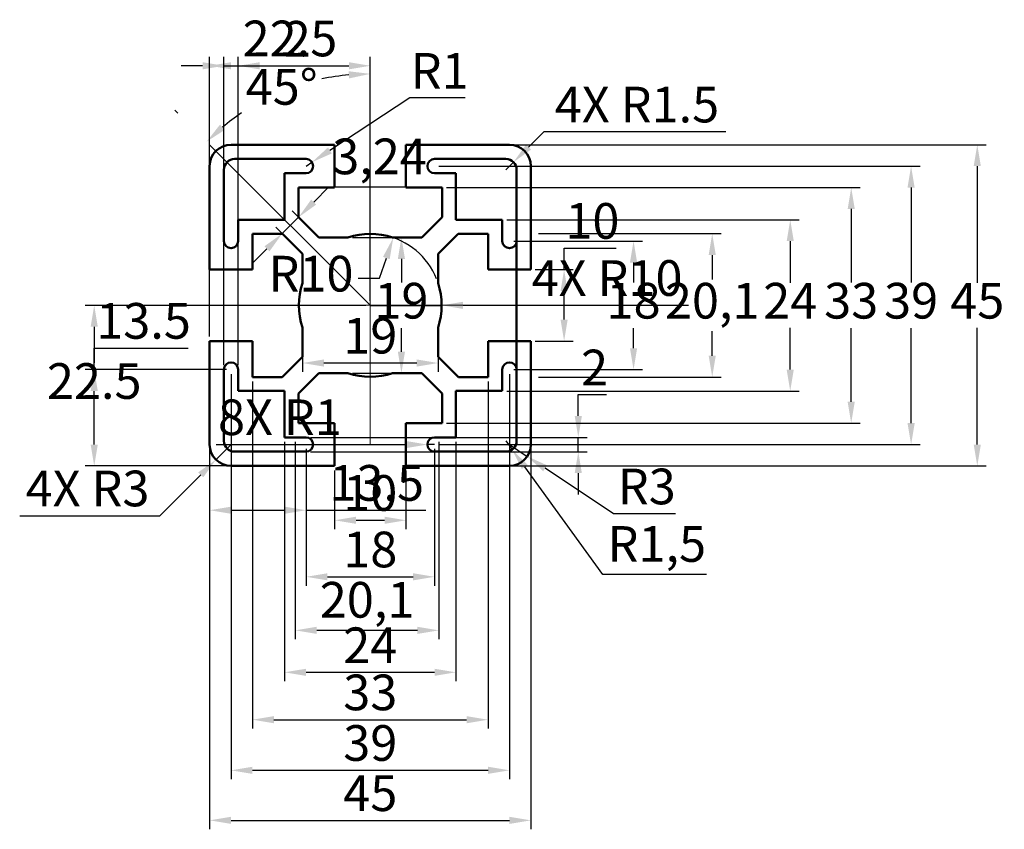
# Model space of a CAD drawing. Units: millimetres. Extents: x 19 to 157, y -26 to 87.
import ezdxf

# ---------------------------------------------------------------- set-up
doc = ezdxf.new("R2010")
doc.units = ezdxf.units.MM
doc.linetypes.add('CENTER', pattern=[50.8, 31.75, -6.35, 6.35, -6.35])
for name, color, linetype, lineweight in [('M-CNTR', 1, 'CENTER', 18), ('M-DIMS', 2, 'Continuous', 25), ('M-OUTL', 7, 'Continuous', 50)]:
    doc.layers.add(name, color=color, linetype=linetype, lineweight=lineweight)
doc.styles.get("Standard").update_dxf_attribs({"font": 'arial.ttf'})
doc.dimstyles.new('ISO-25', dxfattribs={"dimtxt": 5, "dimasz": 3, "dimexe": 1.25, "dimexo": 0.625, "dimtad": 1, "dimtih": 1, "dimtoh": 1, "dimtxsty": 'Standard', "dimcen": 2.5, "dimadec": 0, "dimazin": 0, "dimtfac": 1, "dimtmove": 0, "dimatfit": 3, "dimfxl": 1, "dimarcsym": 0})

# ---------------------------------------------------------------- blocks, each defined once
blk = doc.blocks.new('*D1')
at = {"layer": 'Defpoints', "color": 0, "transparency": 16777216}
for p in [(63.57, 24.73), (73.57, 24.73), (73.57, 17.12)]:
    blk.add_point(p, dxfattribs=at)
at = {"layer": 'M-DIMS', "color": 0, "lineweight": -2, "transparency": 16777216}
for p, q in [((63.57, 24.11), (63.57, 15.87)), ((73.57, 24.11), (73.57, 15.87)), ((66.57, 17.12), (70.57, 17.12))]:
    blk.add_line(p, q, dxfattribs=at)
at = {"layer": 'M-DIMS', "color": 0, "transparency": 16777216}
for points in [[(66.57, 17.62), (66.57, 16.62), (63.57, 17.12)], [(70.57, 17.62), (70.57, 16.62), (73.57, 17.12)]]:
    blk.add_solid(points, dxfattribs=at)
at = {"layer": 'M-DIMS', "color": 0, "transparency": 16777216, "insert": (68.57, 20.3), "char_height": 5, "attachment_point": 5}
blk.add_mtext('10', dxfattribs=at)
blk = doc.blocks.new('*D2')
at = {"layer": 'Defpoints', "color": 0, "transparency": 16777216}
for p in [(59.57, 27.73), (77.57, 27.73), (77.57, 9.2)]:
    blk.add_point(p, dxfattribs=at)
at = {"layer": 'M-DIMS', "color": 0, "lineweight": -2, "transparency": 16777216}
for p, q in [((59.57, 27.11), (59.57, 7.95)), ((77.57, 27.11), (77.57, 7.95)), ((62.57, 9.2), (74.57, 9.2))]:
    blk.add_line(p, q, dxfattribs=at)
at = {"layer": 'M-DIMS', "color": 0, "transparency": 16777216}
for points in [[(62.57, 9.7), (62.57, 8.7), (59.57, 9.2)], [(74.57, 9.7), (74.57, 8.7), (77.57, 9.2)]]:
    blk.add_solid(points, dxfattribs=at)
at = {"layer": 'M-DIMS', "color": 0, "transparency": 16777216, "insert": (68.57, 12.38), "char_height": 5, "attachment_point": 5}
blk.add_mtext('18', dxfattribs=at)
blk = doc.blocks.new('*D3')
at = {"layer": 'Defpoints', "color": 0, "transparency": 16777216}
for p in [(56.57, 28.73), (80.57, 28.73), (80.57, -4.18)]:
    blk.add_point(p, dxfattribs=at)
at = {"layer": 'M-DIMS', "color": 0, "lineweight": -2, "transparency": 16777216}
for p, q in [((56.57, 28.11), (56.57, -5.43)), ((80.57, 28.11), (80.57, -5.43)), ((59.57, -4.18), (77.57, -4.18))]:
    blk.add_line(p, q, dxfattribs=at)
at = {"layer": 'M-DIMS', "color": 0, "transparency": 16777216}
for points in [[(59.57, -3.68), (59.57, -4.68), (56.57, -4.18)], [(77.57, -3.68), (77.57, -4.68), (80.57, -4.18)]]:
    blk.add_solid(points, dxfattribs=at)
at = {"layer": 'M-DIMS', "color": 0, "transparency": 16777216, "insert": (68.57, -1.04), "char_height": 5, "attachment_point": 5}
blk.add_mtext('24', dxfattribs=at)
blk = doc.blocks.new('*D4')
at = {"layer": 'Defpoints', "color": 0, "transparency": 16777216}
for p in [(58.07, 28.73), (78.17, 28.73), (58.07, 1.7)]:
    blk.add_point(p, dxfattribs=at)
at = {"layer": 'M-DIMS', "color": 0, "lineweight": -2, "transparency": 16777216}
for p, q in [((58.07, 28.11), (58.07, 0.45)), ((78.17, 28.11), (78.17, 0.45)), ((75.17, 1.7), (61.07, 1.7))]:
    blk.add_line(p, q, dxfattribs=at)
at = {"layer": 'M-DIMS', "color": 0, "transparency": 16777216}
for points in [[(61.07, 2.2), (61.07, 1.2), (58.07, 1.7)], [(75.17, 2.2), (75.17, 1.2), (78.17, 1.7)]]:
    blk.add_solid(points, dxfattribs=at)
at = {"layer": 'M-DIMS', "color": 0, "transparency": 16777216, "insert": (68.12, 5.33), "char_height": 5, "attachment_point": 5}
blk.add_mtext('20,1', dxfattribs=at)
blk = doc.blocks.new('*D5')
at = {"layer": 'Defpoints', "color": 0, "transparency": 16777216}
for p in [(52.07, 37.18), (85.07, 37.18), (85.07, -10.82)]:
    blk.add_point(p, dxfattribs=at)
at = {"layer": 'M-DIMS', "color": 0, "lineweight": -2, "transparency": 16777216}
for p, q in [((52.07, 36.56), (52.07, -12.07)), ((85.07, 36.56), (85.07, -12.07)), ((55.07, -10.82), (82.07, -10.82))]:
    blk.add_line(p, q, dxfattribs=at)
at = {"layer": 'M-DIMS', "color": 0, "transparency": 16777216}
for points in [[(55.07, -10.32), (55.07, -11.32), (52.07, -10.82)], [(82.07, -10.32), (82.07, -11.32), (85.07, -10.82)]]:
    blk.add_solid(points, dxfattribs=at)
at = {"layer": 'M-DIMS', "color": 0, "transparency": 16777216, "insert": (68.57, -7.64), "char_height": 5, "attachment_point": 5}
blk.add_mtext('33', dxfattribs=at)
blk = doc.blocks.new('*D6')
at = {"layer": 'Defpoints', "color": 0, "transparency": 16777216}
for p in [(49.07, 38.23), (88.07, 38.23), (88.07, -17.91)]:
    blk.add_point(p, dxfattribs=at)
at = {"layer": 'M-DIMS', "color": 0, "lineweight": -2, "transparency": 16777216}
for p, q in [((49.07, 37.61), (49.07, -19.16)), ((88.07, 37.61), (88.07, -19.16)), ((52.07, -17.91), (85.07, -17.91))]:
    blk.add_line(p, q, dxfattribs=at)
at = {"layer": 'M-DIMS', "color": 0, "transparency": 16777216}
for points in [[(52.07, -17.41), (52.07, -18.41), (49.07, -17.91)], [(85.07, -17.41), (85.07, -18.41), (88.07, -17.91)]]:
    blk.add_solid(points, dxfattribs=at)
at = {"layer": 'M-DIMS', "color": 0, "transparency": 16777216, "insert": (68.57, -14.73), "char_height": 5, "attachment_point": 5}
blk.add_mtext('39', dxfattribs=at)
blk = doc.blocks.new('*D7')
at = {"layer": 'Defpoints', "color": 0, "transparency": 16777216}
for p in [(46.07, 27.73), (91.07, 27.73), (91.07, -24.92)]:
    blk.add_point(p, dxfattribs=at)
at = {"layer": 'M-DIMS', "color": 0, "lineweight": -2, "transparency": 16777216}
for p, q in [((46.07, 27.11), (46.07, -26.17)), ((91.07, 27.11), (91.07, -26.17)), ((49.07, -24.92), (88.07, -24.92))]:
    blk.add_line(p, q, dxfattribs=at)
at = {"layer": 'M-DIMS', "color": 0, "transparency": 16777216}
for points in [[(49.07, -24.42), (49.07, -25.42), (46.07, -24.92)], [(88.07, -24.42), (88.07, -25.42), (91.07, -24.92)]]:
    blk.add_solid(points, dxfattribs=at)
at = {"layer": 'M-DIMS', "color": 0, "transparency": 16777216, "insert": (68.57, -21.76), "char_height": 5, "attachment_point": 5}
blk.add_mtext('45', dxfattribs=at)
blk = doc.blocks.new('*D8')
at = {"layer": 'Defpoints', "color": 0, "transparency": 16777216}
for p in [(91.07, 52.23), (95.72, 52.23), (91.07, 42.23)]:
    blk.add_point(p, dxfattribs=at)
at = {"layer": 'M-DIMS', "color": 0, "lineweight": -2, "transparency": 16777216}
for p, q in [((95.72, 52.23), (95.72, 55.23)), ((95.72, 55.23), (103.02, 55.23)), ((91.69, 52.23), (96.97, 52.23)), ((95.72, 45.23), (95.72, 49.23)), ((91.69, 42.23), (96.97, 42.23))]:
    blk.add_line(p, q, dxfattribs=at)
at = {"layer": 'M-DIMS', "color": 0, "transparency": 16777216}
for points in [[(95.22, 49.23), (96.22, 49.23), (95.72, 52.23)], [(95.22, 45.23), (96.22, 45.23), (95.72, 42.23)]]:
    blk.add_solid(points, dxfattribs=at)
at = {"layer": 'M-DIMS', "color": 0, "transparency": 16777216, "insert": (99.68, 58.41), "char_height": 5, "attachment_point": 5}
blk.add_mtext('10', dxfattribs=at)
blk = doc.blocks.new('*D9')
at = {"layer": 'Defpoints', "color": 0, "transparency": 16777216}
for p in [(88.07, 56.23), (105.45, 56.23), (88.07, 38.23)]:
    blk.add_point(p, dxfattribs=at)
at = {"layer": 'M-DIMS', "color": 0, "lineweight": -2, "transparency": 16777216}
for p, q in [((88.69, 56.23), (106.7, 56.23)), ((105.45, 53.23), (105.45, 50.41)), ((105.45, 41.23), (105.45, 44.05)), ((88.69, 38.23), (106.7, 38.23))]:
    blk.add_line(p, q, dxfattribs=at)
at = {"layer": 'M-DIMS', "color": 0, "transparency": 16777216}
for points in [[(104.95, 53.23), (105.95, 53.23), (105.45, 56.23)], [(104.95, 41.23), (105.95, 41.23), (105.45, 38.23)]]:
    blk.add_solid(points, dxfattribs=at)
at = {"layer": 'M-DIMS', "color": 0, "transparency": 16777216, "insert": (105.45, 47.23), "char_height": 5, "attachment_point": 5}
blk.add_mtext('18', dxfattribs=at)
blk = doc.blocks.new('*D10')
at = {"layer": 'Defpoints', "color": 0, "transparency": 16777216}
for p in [(91.51, 57.28), (116.47, 57.28), (91.51, 37.18)]:
    blk.add_point(p, dxfattribs=at)
at = {"layer": 'M-DIMS', "color": 0, "lineweight": -2, "transparency": 16777216}
for p, q in [((92.14, 57.28), (117.72, 57.28)), ((116.47, 54.28), (116.47, 50.86)), ((116.47, 40.18), (116.47, 43.6)), ((92.14, 37.18), (117.72, 37.18))]:
    blk.add_line(p, q, dxfattribs=at)
at = {"layer": 'M-DIMS', "color": 0, "transparency": 16777216}
for points in [[(115.97, 54.28), (116.97, 54.28), (116.47, 57.28)], [(115.97, 40.18), (116.97, 40.18), (116.47, 37.18)]]:
    blk.add_solid(points, dxfattribs=at)
at = {"layer": 'M-DIMS', "color": 0, "transparency": 16777216, "insert": (116.47, 47.23), "char_height": 5, "attachment_point": 5}
blk.add_mtext('20,1', dxfattribs=at)
blk = doc.blocks.new('*D11')
at = {"layer": 'Defpoints', "color": 0, "transparency": 16777216}
for p in [(87.07, 59.23), (127.4, 59.23), (87.07, 35.23)]:
    blk.add_point(p, dxfattribs=at)
at = {"layer": 'M-DIMS', "color": 0, "lineweight": -2, "transparency": 16777216}
for p, q in [((87.69, 59.23), (128.65, 59.23)), ((127.4, 56.23), (127.4, 50.37)), ((127.4, 38.23), (127.4, 44.1)), ((87.69, 35.23), (128.65, 35.23))]:
    blk.add_line(p, q, dxfattribs=at)
at = {"layer": 'M-DIMS', "color": 0, "transparency": 16777216}
for points in [[(126.9, 56.23), (127.9, 56.23), (127.4, 59.23)], [(126.9, 38.23), (127.9, 38.23), (127.4, 35.23)]]:
    blk.add_solid(points, dxfattribs=at)
at = {"layer": 'M-DIMS', "color": 0, "transparency": 16777216, "insert": (127.4, 47.23), "char_height": 5, "attachment_point": 5}
blk.add_mtext('24', dxfattribs=at)
blk = doc.blocks.new('*D12')
at = {"layer": 'Defpoints', "color": 0, "transparency": 16777216}
for p in [(78.62, 63.73), (135.94, 63.73), (78.62, 30.73)]:
    blk.add_point(p, dxfattribs=at)
at = {"layer": 'M-DIMS', "color": 0, "lineweight": -2, "transparency": 16777216}
for p, q in [((79.24, 63.73), (137.19, 63.73)), ((135.94, 60.73), (135.94, 50.41)), ((135.94, 33.73), (135.94, 44.05)), ((79.24, 30.73), (137.19, 30.73))]:
    blk.add_line(p, q, dxfattribs=at)
at = {"layer": 'M-DIMS', "color": 0, "transparency": 16777216}
for points in [[(135.44, 60.73), (136.44, 60.73), (135.94, 63.73)], [(135.44, 33.73), (136.44, 33.73), (135.94, 30.73)]]:
    blk.add_solid(points, dxfattribs=at)
at = {"layer": 'M-DIMS', "color": 0, "transparency": 16777216, "insert": (135.94, 47.23), "char_height": 5, "attachment_point": 5}
blk.add_mtext('33', dxfattribs=at)
blk = doc.blocks.new('*D13')
at = {"layer": 'Defpoints', "color": 0, "transparency": 16777216}
for p in [(77.57, 66.73), (77.57, 27.73), (144.33, 27.73)]:
    blk.add_point(p, dxfattribs=at)
at = {"layer": 'M-DIMS', "color": 0, "lineweight": -2, "transparency": 16777216}
for p, q in [((78.19, 66.73), (145.58, 66.73)), ((144.33, 63.73), (144.33, 50.41)), ((144.33, 30.73), (144.33, 44.05)), ((78.19, 27.73), (145.58, 27.73))]:
    blk.add_line(p, q, dxfattribs=at)
at = {"layer": 'M-DIMS', "color": 0, "transparency": 16777216}
for points in [[(143.83, 63.73), (144.83, 63.73), (144.33, 66.73)], [(143.83, 30.73), (144.83, 30.73), (144.33, 27.73)]]:
    blk.add_solid(points, dxfattribs=at)
at = {"layer": 'M-DIMS', "color": 0, "transparency": 16777216, "insert": (144.33, 47.23), "char_height": 5, "attachment_point": 5}
blk.add_mtext('39', dxfattribs=at)
blk = doc.blocks.new('*D14')
at = {"layer": 'Defpoints', "color": 0, "transparency": 16777216}
for p in [(88.07, 69.73), (88.07, 24.73), (153.6, 24.73)]:
    blk.add_point(p, dxfattribs=at)
at = {"layer": 'M-DIMS', "color": 0, "lineweight": -2, "transparency": 16777216}
for p, q in [((88.69, 69.73), (154.85, 69.73)), ((153.6, 66.73), (153.6, 50.4)), ((153.6, 27.73), (153.6, 44.06)), ((88.69, 24.73), (154.85, 24.73))]:
    blk.add_line(p, q, dxfattribs=at)
at = {"layer": 'M-DIMS', "color": 0, "transparency": 16777216}
for points in [[(153.1, 66.73), (154.1, 66.73), (153.6, 69.73)], [(153.1, 27.73), (154.1, 27.73), (153.6, 24.73)]]:
    blk.add_solid(points, dxfattribs=at)
at = {"layer": 'M-DIMS', "color": 0, "transparency": 16777216, "insert": (153.6, 47.23), "char_height": 5, "attachment_point": 5}
blk.add_mtext('45', dxfattribs=at)
blk = doc.blocks.new('*D15')
at = {"layer": 'Defpoints', "color": 0, "transparency": 16777216}
for p in [(71.79, 56.7), (68.57, 47.23)]:
    blk.add_point(p, dxfattribs=at)
at = {"layer": 'M-DIMS', "color": 0, "lineweight": -2, "transparency": 16777216}
for p, q in [((69.85, 51.02), (70.82, 53.86)), ((66.85, 51.02), (69.85, 51.02))]:
    blk.add_line(p, q, dxfattribs=at)
blk.add_arc((68.57, 47.23), 10, 21.7759, 78.3911, dxfattribs=at)
at = {"layer": 'M-DIMS', "color": 0, "transparency": 16777216}
blk.add_solid([(70.35, 54.02), (71.29, 53.7), (71.79, 56.7)], dxfattribs=at)
at = {"layer": 'M-DIMS', "color": 0, "transparency": 16777216, "insert": (60.26, 51.02), "char_height": 5, "attachment_point": 5}
blk.add_mtext('R10', dxfattribs=at)
blk = doc.blocks.new('*D16')
at = {"layer": 'Defpoints', "color": 0, "transparency": 16777216}
for p in [(65.44, 56.73), (65.44, 37.73), (72.93, 37.73)]:
    blk.add_point(p, dxfattribs=at)
at = {"layer": 'M-DIMS', "color": 0, "lineweight": -2, "transparency": 16777216}
for p, q in [((66.07, 56.73), (74.18, 56.73)), ((72.93, 53.73), (72.93, 50.41)), ((72.93, 40.73), (72.93, 44.05)), ((66.07, 37.73), (74.18, 37.73))]:
    blk.add_line(p, q, dxfattribs=at)
at = {"layer": 'M-DIMS', "color": 0, "transparency": 16777216}
for points in [[(72.43, 53.73), (73.43, 53.73), (72.93, 56.73)], [(72.43, 40.73), (73.43, 40.73), (72.93, 37.73)]]:
    blk.add_solid(points, dxfattribs=at)
at = {"layer": 'M-DIMS', "color": 0, "transparency": 16777216, "insert": (72.93, 47.23), "char_height": 5, "attachment_point": 5}
blk.add_mtext('19', dxfattribs=at)
blk = doc.blocks.new('*D17')
at = {"layer": 'Defpoints', "color": 0, "transparency": 16777216}
for p in [(59.07, 44.11), (78.07, 44.11), (59.07, 39.15)]:
    blk.add_point(p, dxfattribs=at)
at = {"layer": 'M-DIMS', "color": 0, "lineweight": -2, "transparency": 16777216}
for p, q in [((59.07, 43.48), (59.07, 37.9)), ((78.07, 43.48), (78.07, 37.9)), ((75.07, 39.15), (62.07, 39.15))]:
    blk.add_line(p, q, dxfattribs=at)
at = {"layer": 'M-DIMS', "color": 0, "transparency": 16777216}
for points in [[(62.07, 39.65), (62.07, 38.65), (59.07, 39.15)], [(75.07, 39.65), (75.07, 38.65), (78.07, 39.15)]]:
    blk.add_solid(points, dxfattribs=at)
at = {"layer": 'M-DIMS', "color": 0, "transparency": 16777216, "insert": (68.57, 42.33), "char_height": 5, "attachment_point": 5}
blk.add_mtext('19', dxfattribs=at)
blk = doc.blocks.new('*D18')
at = {"layer": 'Defpoints', "color": 0, "transparency": 16777216}
for p in [(58.52, 59.57), (61.36, 56.73), (59.07, 54.44)]:
    blk.add_point(p, dxfattribs=at)
at = {"layer": 'M-DIMS', "color": 0, "lineweight": -2, "transparency": 16777216}
for p, q in [((60.64, 61.69), (62.76, 63.82)), ((62.76, 63.82), (76.35, 63.82)), ((56.23, 57.28), (58.52, 59.57)), ((60.92, 57.17), (57.63, 60.46)), ((58.63, 54.88), (55.34, 58.17)), ((54.1, 55.16), (51.98, 53.04))]:
    blk.add_line(p, q, dxfattribs=at)
at = {"layer": 'M-DIMS', "color": 0, "transparency": 16777216}
for points in [[(60.29, 62.05), (60.99, 61.34), (58.52, 59.57)], [(53.75, 55.51), (54.46, 54.81), (56.23, 57.28)]]:
    blk.add_solid(points, dxfattribs=at)
at = {"layer": 'M-DIMS', "color": 0, "transparency": 16777216, "insert": (69.87, 67.45), "char_height": 5, "attachment_point": 5}
blk.add_mtext('3,24', dxfattribs=at)
blk = doc.blocks.new('*D19')
at = {"layer": 'Defpoints', "color": 0, "transparency": 16777216}
for p in [(60.17, 78.56), (41.21, 74.59), (68.57, 74.16), (68.57, 56.73), (68.57, 47.23)]:
    blk.add_point(p, dxfattribs=at)
at = {"layer": 'M-DIMS', "color": 0, "lineweight": -2, "transparency": 16777216}
blk.add_line((68.57, 74.79), (68.57, 80.91), dxfattribs=at)
for start, end in [(95.3024, 102.0676), (123.8004, 129.6976)]:
    blk.add_arc((68.57, 47.23), 32.43, start, end, dxfattribs=at)
at = {"layer": 'M-DIMS', "color": 0, "transparency": 16777216}
for points in [[(65.55, 80.02), (65.59, 79.02), (68.57, 79.66)], [(48.19, 71.81), (47.52, 72.55), (45.64, 70.16)]]:
    blk.add_solid(points, dxfattribs=at)
at = {"layer": 'M-DIMS', "color": 0, "transparency": 16777216, "insert": (56.16, 77.19), "char_height": 5, "attachment_point": 5}
blk.add_mtext('45°', dxfattribs=at)
blk = doc.blocks.new('*D20')
at = {"layer": 'Defpoints', "color": 0, "transparency": 16777216}
for p in [(59.57, 66.73), (60.4, 67.28)]:
    blk.add_point(p, dxfattribs=at)
at = {"layer": 'M-DIMS', "color": 0, "lineweight": -2, "transparency": 16777216}
for p, q in [((74.12, 76.29), (62.91, 68.93)), ((81.84, 76.29), (74.12, 76.29)), ((59.57, 66.73), (60.4, 67.28))]:
    blk.add_line(p, q, dxfattribs=at)
at = {"layer": 'M-DIMS', "color": 0, "transparency": 16777216}
blk.add_solid([(62.64, 69.35), (63.18, 68.51), (60.4, 67.28)], dxfattribs=at)
at = {"layer": 'M-DIMS', "color": 0, "transparency": 16777216, "insert": (78.29, 79.43), "char_height": 5, "attachment_point": 5}
blk.add_mtext('R1', dxfattribs=at)
blk = doc.blocks.new('*D21')
at = {"layer": 'Defpoints', "color": 0, "transparency": 16777216}
for p in [(88.07, 27.73), (90.56, 26.07)]:
    blk.add_point(p, dxfattribs=at)
at = {"layer": 'M-DIMS', "color": 0, "lineweight": -2, "transparency": 16777216}
for p, q in [((88.07, 27.73), (90.56, 26.07)), ((102.65, 18.03), (93.06, 24.41)), ((111.34, 18.03), (102.65, 18.03))]:
    blk.add_line(p, q, dxfattribs=at)
at = {"layer": 'M-DIMS', "color": 0, "transparency": 16777216}
blk.add_solid([(93.34, 24.82), (92.79, 23.99), (90.56, 26.07)], dxfattribs=at)
at = {"layer": 'M-DIMS', "color": 0, "transparency": 16777216, "insert": (107.3, 21.21), "char_height": 5, "attachment_point": 5}
blk.add_mtext('R3', dxfattribs=at)
blk = doc.blocks.new('*D22')
at = {"layer": 'Defpoints', "color": 0, "transparency": 16777216}
for p in [(87.57, 28.23), (88.45, 27.02)]:
    blk.add_point(p, dxfattribs=at)
at = {"layer": 'M-DIMS', "color": 0, "lineweight": -2, "transparency": 16777216}
for p, q in [((87.57, 28.23), (88.45, 27.02)), ((101.13, 9.52), (90.21, 24.59)), ((115.68, 9.52), (101.13, 9.52))]:
    blk.add_line(p, q, dxfattribs=at)
at = {"layer": 'M-DIMS', "color": 0, "transparency": 16777216}
blk.add_solid([(90.61, 24.88), (89.8, 24.3), (88.45, 27.02)], dxfattribs=at)
at = {"layer": 'M-DIMS', "color": 0, "transparency": 16777216, "insert": (108.71, 13.15), "char_height": 5, "attachment_point": 5}
blk.add_mtext('R1,5', dxfattribs=at)
blk = doc.blocks.new('*D23')
at = {"layer": 'Defpoints', "color": 0, "transparency": 16777216}
for p in [(68.57, 80.79), (68.57, 47.23), (46.07, 42.23)]:
    blk.add_point(p, dxfattribs=at)
at = {"layer": 'M-DIMS', "color": 0, "lineweight": -2, "transparency": 16777216}
for p, q in [((46.07, 42.86), (46.07, 82.04)), ((68.57, 47.86), (68.57, 82.04)), ((49.07, 80.79), (65.57, 80.79))]:
    blk.add_line(p, q, dxfattribs=at)
at = {"layer": 'M-DIMS', "color": 0, "transparency": 16777216}
for points in [[(49.07, 81.29), (49.07, 80.29), (46.07, 80.79)], [(65.57, 81.29), (65.57, 80.29), (68.57, 80.79)]]:
    blk.add_solid(points, dxfattribs=at)
at = {"layer": 'M-DIMS', "color": 0, "transparency": 16777216, "insert": (57.32, 83.97), "char_height": 5, "attachment_point": 5}
blk.add_mtext('22.5', dxfattribs=at)
blk = doc.blocks.new('*D24')
at = {"layer": 'Defpoints', "color": 0, "transparency": 16777216}
for p in [(29.9, 47.23), (68.57, 47.23), (63.57, 24.73)]:
    blk.add_point(p, dxfattribs=at)
at = {"layer": 'M-DIMS', "color": 0, "lineweight": -2, "transparency": 16777216}
for p, q in [((67.94, 47.23), (28.65, 47.23)), ((29.9, 44.23), (29.9, 39.16)), ((29.9, 27.73), (29.9, 32.8)), ((62.94, 24.73), (28.65, 24.73))]:
    blk.add_line(p, q, dxfattribs=at)
at = {"layer": 'M-DIMS', "color": 0, "transparency": 16777216}
for points in [[(29.4, 44.23), (30.4, 44.23), (29.9, 47.23)], [(29.4, 27.73), (30.4, 27.73), (29.9, 24.73)]]:
    blk.add_solid(points, dxfattribs=at)
at = {"layer": 'M-DIMS', "color": 0, "transparency": 16777216, "insert": (29.9, 35.98), "char_height": 5, "attachment_point": 5}
blk.add_mtext('22.5', dxfattribs=at)
blk = doc.blocks.new('*D25')
at = {"layer": 'Defpoints', "color": 0, "transparency": 16777216}
for p in [(50.07, 80.79), (48.07, 38.23), (50.07, 38.23)]:
    blk.add_point(p, dxfattribs=at)
at = {"layer": 'M-DIMS', "color": 0, "lineweight": -2, "transparency": 16777216}
for p, q in [((48.07, 38.86), (48.07, 82.04)), ((50.07, 38.86), (50.07, 82.04)), ((45.07, 80.79), (42.07, 80.79)), ((48.07, 80.79), (50.07, 80.79)), ((53.07, 80.79), (60.63, 80.79))]:
    blk.add_line(p, q, dxfattribs=at)
at = {"layer": 'M-DIMS', "color": 0, "transparency": 16777216}
for points in [[(45.07, 81.29), (45.07, 80.29), (48.07, 80.79)], [(53.07, 81.29), (53.07, 80.29), (50.07, 80.79)]]:
    blk.add_solid(points, dxfattribs=at)
at = {"layer": 'M-DIMS', "color": 0, "transparency": 16777216, "insert": (58.35, 83.92), "char_height": 5, "attachment_point": 5}
blk.add_mtext('2', dxfattribs=at)
blk = doc.blocks.new('*D26')
at = {"layer": 'Defpoints', "color": 0, "transparency": 16777216}
for p in [(59.57, 28.73), (97.71, 28.73), (59.57, 26.73)]:
    blk.add_point(p, dxfattribs=at)
at = {"layer": 'M-DIMS', "color": 0, "lineweight": -2, "transparency": 16777216}
for p, q in [((97.71, 31.73), (97.71, 34.73)), ((97.71, 34.73), (101.65, 34.73)), ((60.19, 28.73), (98.96, 28.73)), ((97.71, 26.73), (97.71, 28.73)), ((60.19, 26.73), (98.96, 26.73)), ((97.71, 23.73), (97.71, 20.73))]:
    blk.add_line(p, q, dxfattribs=at)
at = {"layer": 'M-DIMS', "color": 0, "transparency": 16777216}
for points in [[(97.21, 31.73), (98.21, 31.73), (97.71, 28.73)], [(97.21, 23.73), (98.21, 23.73), (97.71, 26.73)]]:
    blk.add_solid(points, dxfattribs=at)
at = {"layer": 'M-DIMS', "color": 0, "transparency": 16777216, "insert": (99.99, 37.87), "char_height": 5, "attachment_point": 5}
blk.add_mtext('2', dxfattribs=at)
blk = doc.blocks.new('*D27')
at = {"layer": 'Defpoints', "color": 0, "transparency": 16777216}
for p in [(46.07, 27.73), (59.57, 27.73), (59.57, 18.53)]:
    blk.add_point(p, dxfattribs=at)
at = {"layer": 'M-DIMS', "color": 0, "lineweight": -2, "transparency": 16777216}
for p, q in [((46.07, 27.11), (46.07, 17.28)), ((59.57, 27.11), (59.57, 17.28)), ((49.07, 18.53), (56.57, 18.53)), ((59.57, 18.53), (76.37, 18.53))]:
    blk.add_line(p, q, dxfattribs=at)
at = {"layer": 'M-DIMS', "color": 0, "transparency": 16777216}
for points in [[(49.07, 19.03), (49.07, 18.03), (46.07, 18.53)], [(56.57, 19.03), (56.57, 18.03), (59.57, 18.53)]]:
    blk.add_solid(points, dxfattribs=at)
at = {"layer": 'M-DIMS', "color": 0, "transparency": 16777216, "insert": (69.47, 21.71), "char_height": 5, "attachment_point": 5}
blk.add_mtext('13.5', dxfattribs=at)
blk = doc.blocks.new('*D28')
at = {"layer": 'Defpoints', "color": 0, "transparency": 16777216}
for p in [(29.9, 38.23), (49.07, 38.23), (49.07, 24.73)]:
    blk.add_point(p, dxfattribs=at)
at = {"layer": 'M-DIMS', "color": 0, "lineweight": -2, "transparency": 16777216}
for p, q in [((29.9, 38.23), (29.9, 41.23)), ((29.9, 41.23), (43.08, 41.23)), ((48.44, 38.23), (28.65, 38.23)), ((29.9, 27.73), (29.9, 35.23)), ((48.44, 24.73), (28.65, 24.73))]:
    blk.add_line(p, q, dxfattribs=at)
at = {"layer": 'M-DIMS', "color": 0, "transparency": 16777216}
for points in [[(29.4, 35.23), (30.4, 35.23), (29.9, 38.23)], [(29.4, 27.73), (30.4, 27.73), (29.9, 24.73)]]:
    blk.add_solid(points, dxfattribs=at)
at = {"layer": 'M-DIMS', "color": 0, "transparency": 16777216, "insert": (36.81, 44.41), "char_height": 5, "attachment_point": 5}
blk.add_mtext('13.5', dxfattribs=at)
blk = doc.blocks.new('*D29')
at = {"layer": 'Defpoints', "color": 0, "transparency": 16777216}
for p in [(68.57, 47.23), (78.57, 47.23)]:
    blk.add_point(p, dxfattribs=at)
at = {"layer": 'M-DIMS', "color": 0, "lineweight": -2, "transparency": 16777216}
for p, q in [((68.57, 47.23), (78.57, 47.23)), ((89.67, 47.23), (81.57, 47.23)), ((113.17, 47.23), (89.67, 47.23))]:
    blk.add_line(p, q, dxfattribs=at)
at = {"layer": 'M-DIMS', "color": 0, "transparency": 16777216}
blk.add_solid([(81.57, 47.73), (81.57, 46.73), (78.57, 47.23)], dxfattribs=at)
at = {"layer": 'M-DIMS', "color": 0, "transparency": 16777216, "insert": (101.74, 50.41), "char_height": 5, "attachment_point": 5}
blk.add_mtext('4X R10', dxfattribs=at)
blk = doc.blocks.new('*D30')
at = {"layer": 'Defpoints', "color": 0, "transparency": 16777216}
for p in [(49.07, 27.73), (46.95, 25.61)]:
    blk.add_point(p, dxfattribs=at)
at = {"layer": 'M-DIMS', "color": 0, "lineweight": -2, "transparency": 16777216}
for p, q in [((49.07, 27.73), (46.95, 25.61)), ((39.09, 17.76), (44.82, 23.49)), ((19.46, 17.76), (39.09, 17.76))]:
    blk.add_line(p, q, dxfattribs=at)
at = {"layer": 'M-DIMS', "color": 0, "transparency": 16777216}
blk.add_solid([(44.47, 23.84), (45.18, 23.14), (46.95, 25.61)], dxfattribs=at)
at = {"layer": 'M-DIMS', "color": 0, "transparency": 16777216, "insert": (28.96, 20.93), "char_height": 5, "attachment_point": 5}
blk.add_mtext('4X R3', dxfattribs=at)
blk = doc.blocks.new('*D31')
at = {"layer": 'Defpoints', "color": 0, "transparency": 16777216}
for p in [(87.57, 66.23), (88.63, 67.29)]:
    blk.add_point(p, dxfattribs=at)
at = {"layer": 'M-DIMS', "color": 0, "lineweight": -2, "transparency": 16777216}
for p, q in [((92.87, 71.54), (90.75, 69.41)), ((118.37, 71.54), (92.87, 71.54)), ((87.57, 66.23), (88.63, 67.29))]:
    blk.add_line(p, q, dxfattribs=at)
at = {"layer": 'M-DIMS', "color": 0, "transparency": 16777216}
blk.add_solid([(90.4, 69.77), (91.1, 69.06), (88.63, 67.29)], dxfattribs=at)
at = {"layer": 'M-DIMS', "color": 0, "transparency": 16777216, "insert": (105.93, 74.71), "char_height": 5, "attachment_point": 5}
blk.add_mtext('4X R1.5', dxfattribs=at)
blk = doc.blocks.new('*D32')
at = {"layer": 'Defpoints', "color": 0, "transparency": 16777216}
for p in [(76.57, 27.73), (77.57, 27.73)]:
    blk.add_point(p, dxfattribs=at)
at = {"layer": 'M-DIMS', "color": 0, "lineweight": -2, "transparency": 16777216}
for p, q in [((46.99, 27.73), (65.46, 27.73)), ((65.46, 27.73), (73.57, 27.73)), ((77.57, 27.73), (76.57, 27.73))]:
    blk.add_line(p, q, dxfattribs=at)
at = {"layer": 'M-DIMS', "color": 0, "transparency": 16777216}
blk.add_solid([(73.57, 28.23), (73.57, 27.23), (76.57, 27.73)], dxfattribs=at)
at = {"layer": 'M-DIMS', "color": 0, "transparency": 16777216, "insert": (55.91, 30.9), "char_height": 5, "attachment_point": 5}
blk.add_mtext('8X R1', dxfattribs=at)

msp = doc.modelspace()

# ---------------------------------------------------------------- linework, layer by layer
at = {"layer": 'M-CNTR'}
for p, q in [((68.567, 47.232), (41.21, 74.589)), ((68.567, 56.732), (68.567, 74.162)), ((68.567, 47.232), (68.567, 57.232)), ((68.567, 47.232), (36.104, 47.232)), ((68.567, 47.232), (68.567, 27.643)), ((68.567, 47.232), (91.514, 47.232))]:
    msp.add_line(p, q, dxfattribs=at)
at = {"layer": 'M-OUTL'}
for p, q in [((63.567, 69.732), (49.067, 69.732)), ((63.567, 63.732), (63.567, 69.732)), ((88.067, 69.732), (73.567, 69.732)), ((73.567, 63.732), (73.567, 69.732)), ((59.567, 67.732), (49.567, 67.732)), ((77.567, 67.732), (87.567, 67.732)), ((46.067, 66.732), (46.067, 52.232)), ((48.067, 56.232), (48.067, 66.232)), ((89.067, 56.232), (89.067, 66.232)), ((91.067, 52.232), (91.067, 66.732)), ((56.567, 59.232), (56.567, 65.732)), ((59.567, 65.732), (56.567, 65.732)), ((77.567, 65.732), (80.567, 65.732)), ((80.567, 63.732), (80.567, 65.732)), ((58.517, 62.181), (58.517, 63.732)), ((59.567, 63.732), (58.517, 63.732)), ((63.567, 63.732), (59.567, 63.732)), ((77.567, 63.732), (73.567, 63.732)), ((77.567, 63.732), (78.617, 63.732)), ((78.617, 59.574), (78.617, 63.732)), ((80.567, 59.232), (80.567, 63.732)), ((58.517, 59.574), (58.517, 62.181)), ((61.358, 56.732), (58.517, 59.574)), ((75.776, 56.732), (78.617, 59.574)), ((56.567, 59.232), (50.067, 59.232)), ((50.067, 56.232), (50.067, 59.232)), ((80.567, 59.232), (85.067, 59.232)), ((85.067, 59.232), (87.067, 59.232)), ((87.067, 56.232), (87.067, 59.232)), ((56.276, 57.232), (52.067, 57.232)), ((52.067, 56.232), (52.067, 57.232)), ((59.067, 54.441), (56.276, 57.232)), ((61.358, 56.732), (65.445, 56.732)), ((71.69, 56.732), (75.776, 56.732)), ((78.067, 54.441), (80.858, 57.232)), ((80.858, 57.232), (85.067, 57.232)), ((85.067, 56.232), (85.067, 57.232)), ((89.067, 37.182), (89.067, 57.282)), ((89.067, 57.282), (89.067, 57.282)), ((52.067, 56.232), (52.067, 52.232)), ((85.067, 52.232), (85.067, 56.232)), ((59.067, 50.355), (59.067, 54.441)), ((78.067, 54.441), (78.067, 50.355)), ((52.067, 52.232), (46.067, 52.232)), ((85.067, 52.232), (91.067, 52.232)), ((59.067, 40.024), (59.067, 44.11)), ((78.067, 44.11), (78.067, 40.024)), ((46.067, 42.232), (46.067, 27.732)), ((52.067, 42.232), (46.067, 42.232)), ((52.067, 42.232), (52.067, 37.182)), ((85.067, 37.182), (85.067, 42.232)), ((85.067, 42.232), (91.067, 42.232)), ((91.067, 27.732), (91.067, 42.232)), ((59.067, 40.024), (56.276, 37.232)), ((78.067, 40.024), (80.858, 37.232)), ((48.067, 38.232), (48.067, 28.232)), ((50.067, 38.232), (50.067, 35.232)), ((61.358, 37.732), (58.517, 34.891)), ((65.445, 37.732), (61.358, 37.732)), ((75.776, 37.732), (71.69, 37.732)), ((75.776, 37.732), (78.617, 34.891)), ((87.067, 38.232), (87.067, 35.232)), ((89.067, 38.232), (89.067, 28.232)), ((56.226, 37.182), (52.067, 37.182)), ((56.276, 37.232), (56.226, 37.182)), ((80.858, 37.232), (80.908, 37.182)), ((80.908, 37.182), (85.067, 37.182)), ((56.567, 35.232), (50.067, 35.232)), ((56.567, 35.232), (56.567, 28.732)), ((58.517, 34.891), (58.517, 30.732)), ((78.617, 34.891), (78.617, 30.732)), ((80.567, 30.732), (80.567, 35.232)), ((80.567, 35.232), (87.067, 35.232)), ((59.567, 30.732), (58.517, 30.732)), ((59.567, 30.732), (63.567, 30.732)), ((59.567, 30.732), (63.567, 30.732)), ((63.567, 30.732), (63.567, 24.732)), ((73.567, 30.732), (77.567, 30.732)), ((73.567, 30.732), (73.567, 24.732)), ((73.567, 30.732), (77.567, 30.732)), ((78.617, 30.732), (77.567, 30.732)), ((80.567, 30.732), (80.567, 28.732)), ((59.567, 28.732), (56.567, 28.732)), ((58.067, 28.732), (59.567, 28.732)), ((77.567, 28.732), (80.567, 28.732)), ((77.567, 28.732), (78.167, 28.732)), ((59.567, 26.732), (49.567, 26.732)), ((77.567, 26.732), (87.567, 26.732)), ((49.067, 24.732), (63.567, 24.732)), ((73.567, 24.732), (88.067, 24.732))]:
    msp.add_line(p, q, dxfattribs=at)
for centre, radius, start, end in [((49.067, 66.732), 3, 90, 180), ((88.067, 66.732), 3, 0, 90), ((49.567, 66.232), 1.5, 90, 180), ((59.567, 66.732), 1, 270, 90), ((77.567, 66.732), 1, 90, 270), ((87.567, 66.232), 1.5, 0, 90), ((68.567, 47.232), 10, 71.80513, 108.19487), ((49.067, 56.232), 1, 180, 0), ((88.067, 56.232), 1, 180, 0), ((68.567, 47.232), 10, 161.80513, 198.19487), ((68.567, 47.232), 10, 341.80513, 18.19487), ((49.067, 38.232), 1, 0, 180), ((88.067, 38.232), 1, 0, 180), ((68.567, 47.232), 10, 251.80513, 288.19487), ((49.067, 27.732), 3, 180, 270), ((49.567, 28.232), 1.5, 180, 270), ((59.567, 27.732), 1, 270, 90), ((77.567, 27.732), 1, 90, 270), ((87.567, 28.232), 1.5, 270, 0), ((88.067, 27.732), 3, 270, 0)]:
    msp.add_arc(centre, radius, start, end, dxfattribs=at)

# ---------------------------------------------------------------- dimensions: what is measured, and where the dimension line sits
at = {"layer": 'M-DIMS'}
for base, p1, p2, override, picture, middle in [((50.067, 80.789), (48.067, 38.232), (50.067, 38.232), {"dimdec": 0, "dimlfac": 1, "dimrnd": 0, "dimzin": 0, "dimdsep": 46, "dimlunit": 2}, '*D25', (58.348, 83.925)), ((68.567, 80.789), (46.067, 42.232), (68.567, 47.232), {"dimdec": 1, "dimlfac": 1, "dimrnd": 0, "dimzin": 0, "dimdsep": 46, "dimlunit": 2}, '*D23', (57.317, 83.967)), ((59.067, 39.148), (78.067, 44.11), (59.067, 44.11), {"dimclrd": 0, "dimclre": 0, "dimclrt": 0}, '*D17', (68.567, 42.326)), ((88.067, -17.906), (49.067, 38.232), (88.067, 38.232), {"dimclrd": 0, "dimclre": 0, "dimclrt": 0}, '*D6', (68.567, -14.726)), ((85.067, -10.821), (52.067, 37.182), (85.067, 37.182), {"dimclrd": 0, "dimclre": 0, "dimclrt": 0}, '*D5', (68.567, -7.642)), ((91.067, -24.924), (46.067, 27.732), (91.067, 27.732), {"dimclrd": 0, "dimclre": 0, "dimclrt": 0}, '*D7', (68.567, -21.756)), ((59.567, 18.532), (46.067, 27.732), (59.567, 27.732), {"dimdec": 1, "dimlfac": 1, "dimrnd": 0, "dimzin": 0, "dimdsep": 46, "dimlunit": 2}, '*D27', (69.47, 21.712)), ((80.567, -4.176), (56.567, 28.732), (80.567, 28.732), {"dimclrd": 0, "dimclre": 0, "dimclrt": 0}, '*D3', (68.567, -1.041)), ((58.067, 1.702), (78.167, 28.732), (58.067, 28.732), {"dimclrd": 0, "dimclre": 0, "dimclrt": 0}, '*D4', (68.117, 5.332)), ((77.567, 9.201), (59.567, 27.732), (77.567, 27.732), {"dimclrd": 0, "dimclre": 0, "dimclrt": 0}, '*D2', (68.567, 12.378)), ((73.567, 17.123), (63.567, 24.732), (73.567, 24.732), {"dimclrd": 0, "dimclre": 0, "dimclrt": 0}, '*D1', (68.567, 20.301))]:
    dim = msp.add_linear_dim(base=base, p1=p1, p2=p2, dimstyle='ISO-25', override=override, dxfattribs=at)
    dim.commit()
    dim.dimension.update_dxf_attribs({"geometry": picture, "text_midpoint": middle})
for center, mpoint, picture, middle in [((59.567, 66.732), (60.403, 67.282), '*D20', (78.295, 76.293)), ((68.567, 47.232), (71.785, 56.701), '*D15', (60.264, 51.02)), ((87.567, 28.232), (88.447, 27.018), '*D22', (108.714, 9.523)), ((88.067, 27.732), (90.565, 26.07), '*D21', (107.304, 18.028))]:
    dim = msp.add_radius_dim(center=center, mpoint=mpoint, dimstyle='ISO-25', override={"dimclrd": 0, "dimclre": 0, "dimclrt": 0}, dxfattribs=at)
    dim.commit()
    dim.dimension.update_dxf_attribs({"geometry": picture, "text_midpoint": middle, "dimtype": 164})
for center, mpoint, text, override, picture, middle in [((87.567, 66.232), (88.628, 67.293), '4X <>', {"dimdec": 1, "dimlfac": 1, "dimrnd": 0, "dimzin": 0, "dimdsep": 46, "dimlunit": 2}, '*D31', (105.931, 74.713)), ((68.567, 47.232), (78.567, 47.232), '4X <>', {"dimdec": 0, "dimlfac": 1, "dimrnd": 0, "dimzin": 0, "dimdsep": 46, "dimlunit": 2}, '*D29', (101.736, 50.409)), ((77.567, 27.732), (76.567, 27.732), '8X <>', {"dimdec": 0, "dimlfac": 1, "dimrnd": 0, "dimzin": 0, "dimdsep": 46, "dimlunit": 2}, '*D32', (55.913, 30.905)), ((49.067, 27.732), (46.946, 25.611), '4X <>', {"dimdec": 0, "dimlfac": 1, "dimrnd": 0, "dimzin": 0, "dimdsep": 46, "dimlunit": 2}, '*D30', (28.962, 20.935))]:
    dim = msp.add_radius_dim(center=center, mpoint=mpoint, text=text, dimstyle='ISO-25', override=override, dxfattribs=at)
    dim.commit()
    dim.dimension.update_dxf_attribs({"geometry": picture, "text_midpoint": middle})
dim = msp.add_angular_dim_2l(base=(60.174, 78.556), line1=((68.567, 56.732), (68.567, 74.162)), line2=((68.567, 47.232), (41.21, 74.589)), dimstyle='ISO-25', override={"dimclrd": 0, "dimclre": 0, "dimclrt": 0}, dxfattribs=at)
dim.commit()
dim.dimension.update_dxf_attribs({"geometry": '*D19', "text_midpoint": (56.157, 77.192)})
for p1, p2, distance, picture, middle in [((59.067, 54.441), (61.358, 56.732), 4.018, '*D18', (69.867, 67.446)), ((65.445, 56.732), (65.445, 37.732), 7.489, '*D16', (72.934, 47.232))]:
    dim = msp.add_aligned_dim(p1=p1, p2=p2, distance=distance, dimstyle='ISO-25', override={"dimclrd": 0, "dimclre": 0, "dimclrt": 0}, dxfattribs=at)
    dim.commit()
    dim.dimension.update_dxf_attribs({"geometry": picture, "text_midpoint": middle})
for base, p1, p2, override, picture, middle in [((153.6, 24.732), (88.067, 69.732), (88.067, 24.732), {"dimclrd": 0, "dimclre": 0, "dimclrt": 0}, '*D14', (153.6, 47.232)), ((144.326, 27.732), (77.567, 66.732), (77.567, 27.732), {"dimclrd": 0, "dimclre": 0, "dimclrt": 0}, '*D13', (144.326, 47.232)), ((135.945, 63.732), (78.617, 30.732), (78.617, 63.732), {"dimclrd": 0, "dimclre": 0, "dimclrt": 0}, '*D12', (135.945, 47.232)), ((95.72, 52.232), (91.067, 42.232), (91.067, 52.232), {"dimclrd": 0, "dimclre": 0, "dimclrt": 0}, '*D8', (99.682, 58.41)), ((127.395, 59.232), (87.067, 35.232), (87.067, 59.232), {"dimclrd": 0, "dimclre": 0, "dimclrt": 0}, '*D11', (127.395, 47.232)), ((116.472, 57.282), (91.514, 37.182), (91.514, 57.282), {"dimclrd": 0, "dimclre": 0, "dimclrt": 0}, '*D10', (116.472, 47.232)), ((105.447, 56.232), (88.067, 38.232), (88.067, 56.232), {"dimclrd": 0, "dimclre": 0, "dimclrt": 0}, '*D9', (105.447, 47.232)), ((29.904, 47.232), (63.567, 24.732), (68.567, 47.232), {"dimdec": 1, "dimlfac": 1, "dimrnd": 0, "dimzin": 0, "dimdsep": 46, "dimlunit": 2}, '*D24', (29.904, 35.982)), ((29.904, 38.232), (49.067, 24.732), (49.067, 38.232), {"dimdec": 1, "dimlfac": 1, "dimrnd": 0, "dimzin": 0, "dimdsep": 46, "dimlunit": 2}, '*D28', (36.806, 44.412)), ((97.714, 28.732), (59.567, 26.732), (59.567, 28.732), {"dimdec": 0, "dimlfac": 1, "dimrnd": 0, "dimzin": 0, "dimdsep": 46, "dimlunit": 2}, '*D26', (99.995, 37.868))]:
    dim = msp.add_linear_dim(base=base, p1=p1, p2=p2, angle=90, dimstyle='ISO-25', override=override, dxfattribs=at)
    dim.commit()
    dim.dimension.update_dxf_attribs({"geometry": picture, "text_midpoint": middle})

doc.saveas('drawing.dxf')
